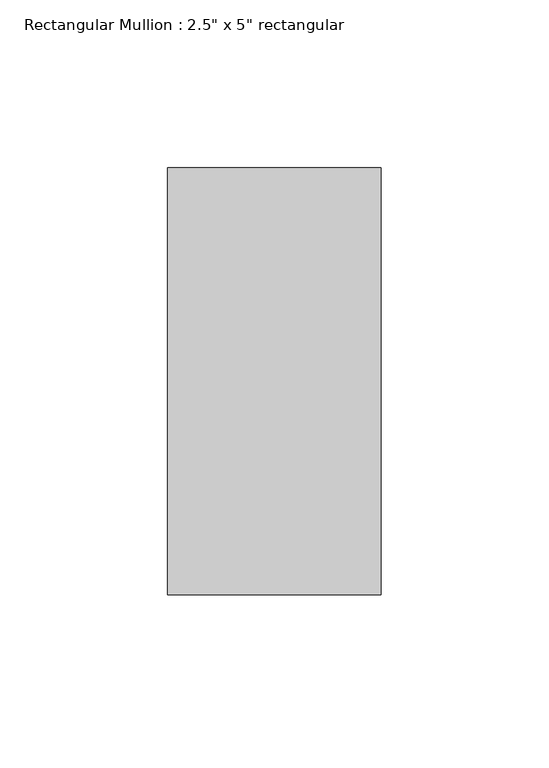
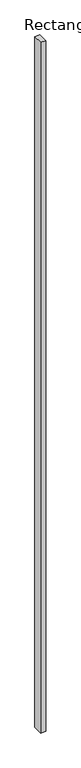
"""IFC4 building model written with IfcOpenShell, lengths in millimetres: member geometry."""

from ifc_helpers import new_model, si_unit, frame, origin, place, context, project, spatial, polyline, outline, extrude, source, transform, mapped, element, save


def member_1c0fec03(model_context):
    return source(origin(), model_context, "Body", "SweptSolid", [
        extrude(outline(polyline([(0.0, 63.5), (0.0, -63.5), (-63.5, -63.5), (-63.5, 63.5), (0.0, 63.5)])), frame((0.0, 0.0, -9213.85), z_axis=(0.0, 0.0, 1.0), x_axis=(1.0, 0.0, 0.0)), (0.0, 0.0, 1.0), 9213.85),
    ])


if __name__ == "__main__":
    model = new_model("IFC4")
    model_context = context("Model", 3, world=origin())
    ifc_project = project(units=[si_unit("LENGTHUNIT", "METRE", prefix="MILLI")], contexts=[model_context])
    site = spatial("IfcSite", under=ifc_project)
    building = spatial("IfcBuilding", under=site)
    placement = place(None, origin())
    member_shape = member_1c0fec03(model_context)
    element("IfcMember", 1, ObjectType="Rectangular Mullion : 2.5\" x 5\" rectangular", at=placement, inside=building, context=model_context, shape_type="MappedRepresentation", body=[
        mapped(member_shape, transform((0.0, 0.0, 0.0), x_axis=(1.0, 0.0, 0.0), y_axis=(0.0, 1.0, 0.0), z_axis=(0.0, 0.0, 1.0))),
    ])
    save(model, "model.ifc")

# Revit data of these elements
# Type "Rectangular Mullion : 2.5\" x 5\" rectangular"
#   built-in parameter 1007304 = 0.416667 (stored number, unit not read)
#   built-in parameter 1007301 = 0.104167 (stored number, unit not read)
#   built-in parameter 1007300 = 0.104167 (stored number, unit not read)
# Element 1 (IfcMember, "Rectangular Mullion : 2.5\" x 5\" rectangular")
#   Materials on its faces: "Aluminum"
# Materials
#   "Aluminum": class "Metal", colour RGB 247 247 247, transparency 0, Description = "Aluminum 6061", Cost = 0
